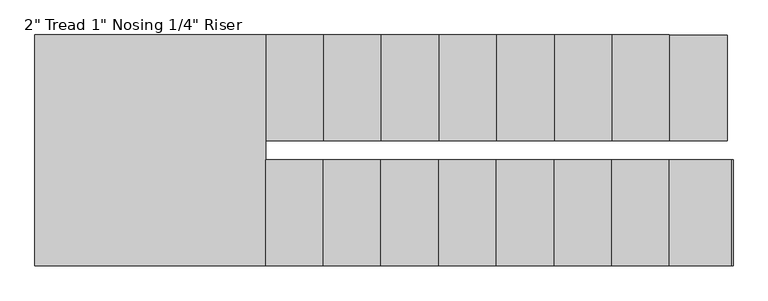
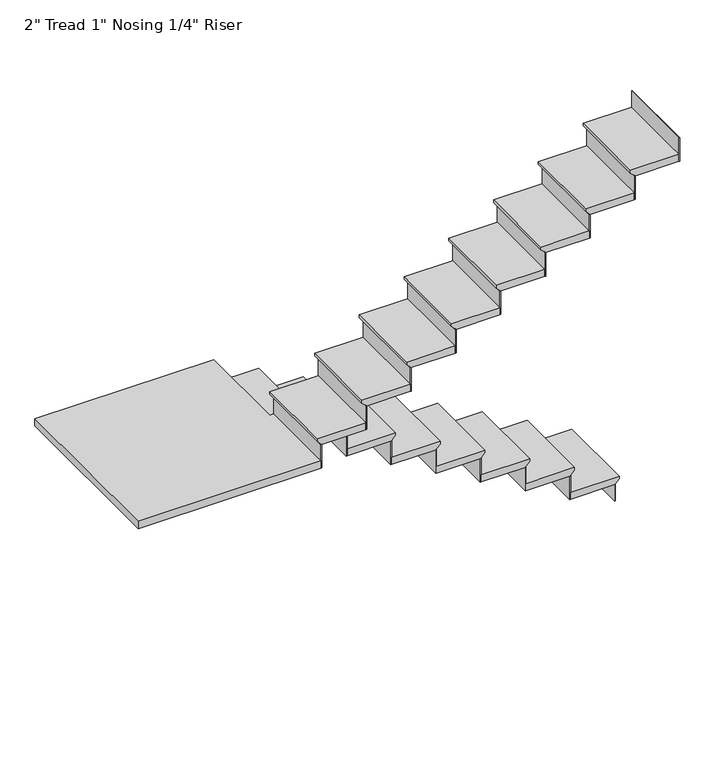
"""IFC4 building model written with IfcOpenShell, lengths in millimetres: stair flight geometry."""

from ifc_helpers import new_model, si_unit, origin, place, context, project, spatial, faceted_brep, source, transform, mapped, element, save


def stair_flight_d84c00c9(model_context):
    return source(origin(), model_context, "Body", "Brep", [
        faceted_brep([(-1805.9198569, -5306.3933037, 9751.4833333), (-1805.9198569, -5306.3933037, 9770.5333333), (-1805.9198569, -5865.1933037, 9770.5333333), (-1805.9198569, -5865.1933037, 9751.4833333), (-1831.3198569, -5306.3933037, 9726.0833333), (-1831.3198569, -5865.1933037, 9726.0833333), (-2136.1198569, -5306.3933037, 9770.5333333), (-2136.1198569, -5865.1933037, 9770.5333333), (-1831.3198569, -5865.1933037, 9719.7333333), (-2136.1198569, -5865.1933037, 9719.7333333), (-2136.1198569, -5306.3933037, 9719.7333333), (-1831.3198569, -5306.3933037, 9719.7333333)], [[[0, 1, 2, 3]], [[4, 0, 3, 5]], [[2, 1, 6, 7]], [[8, 9, 10, 11]], [[2, 7, 9, 8, 5, 3]], [[8, 11, 4, 5]], [[6, 1, 0, 4, 11, 10]], [[7, 6, 10, 9]]]),
        faceted_brep([(-1831.3198569, -5306.3933037, 9719.7333333), (-1831.3198569, -5306.3933037, 9601.2), (-1837.6698569, -5306.3933037, 9601.2), (-1837.6698569, -5306.3933037, 9719.7333333), (-1831.3198569, -5865.1933037, 9719.7333333), (-1837.6698569, -5865.1933037, 9719.7333333), (-1837.6698569, -5865.1933037, 9601.2), (-1831.3198569, -5865.1933037, 9601.2)], [[[0, 1, 2, 3]], [[4, 5, 6, 7]], [[1, 0, 4, 7]], [[2, 1, 7, 6]], [[3, 2, 6, 5]], [[0, 3, 5, 4]]]),
        faceted_brep([(-2136.1198569, -5306.3933037, 9889.0666667), (-2136.1198569, -5306.3933037, 9719.7333333), (-2142.4698569, -5306.3933037, 9719.7333333), (-2142.4698569, -5306.3933037, 9889.0666667), (-2136.1198569, -5865.1933037, 9889.0666667), (-2142.4698569, -5865.1933037, 9889.0666667), (-2142.4698569, -5865.1933037, 9719.7333333), (-2136.1198569, -5865.1933037, 9719.7333333)], [[[0, 1, 2, 3]], [[4, 5, 6, 7]], [[1, 0, 4, 7]], [[2, 1, 7, 6]], [[3, 2, 6, 5]], [[0, 3, 5, 4]]]),
        faceted_brep([(-2110.7198569, -5865.1933037, 9939.8666667), (-2110.7198569, -5306.3933037, 9939.8666667), (-2440.9198569, -5306.3933037, 9939.8666667), (-2440.9198569, -5865.1933037, 9939.8666667), (-2136.1198569, -5865.1933037, 9889.0666667), (-2440.9198569, -5865.1933037, 9889.0666667), (-2440.9198569, -5306.3933037, 9889.0666667), (-2136.1198569, -5306.3933037, 9889.0666667), (-2136.1198569, -5865.1933037, 9895.4166667), (-2110.7198569, -5865.1933037, 9920.8166667), (-2136.1198569, -5306.3933037, 9895.4166667), (-2110.7198569, -5306.3933037, 9920.8166667)], [[[0, 1, 2, 3]], [[4, 5, 6, 7]], [[0, 3, 5, 4, 8, 9]], [[4, 7, 10, 8]], [[2, 1, 11, 10, 7, 6]], [[3, 2, 6, 5]], [[11, 1, 0, 9]], [[10, 11, 9, 8]]]),
        faceted_brep([(-2440.9198569, -5306.3933037, 10058.4), (-2440.9198569, -5306.3933037, 9889.0666667), (-2447.2698569, -5306.3933037, 9889.0666667), (-2447.2698569, -5306.3933037, 10058.4), (-2440.9198569, -5865.1933037, 10058.4), (-2447.2698569, -5865.1933037, 10058.4), (-2447.2698569, -5865.1933037, 9889.0666667), (-2440.9198569, -5865.1933037, 9889.0666667)], [[[0, 1, 2, 3]], [[4, 5, 6, 7]], [[1, 0, 4, 7]], [[2, 1, 7, 6]], [[3, 2, 6, 5]], [[0, 3, 5, 4]]]),
        faceted_brep([(-2415.5198569, -5865.1933037, 10109.2), (-2415.5198569, -5306.3933037, 10109.2), (-2745.7198569, -5306.3933037, 10109.2), (-2745.7198569, -5865.1933037, 10109.2), (-2440.9198569, -5865.1933037, 10058.4), (-2745.7198569, -5865.1933037, 10058.4), (-2745.7198569, -5306.3933037, 10058.4), (-2440.9198569, -5306.3933037, 10058.4), (-2440.9198569, -5865.1933037, 10064.75), (-2415.5198569, -5865.1933037, 10090.15), (-2440.9198569, -5306.3933037, 10064.75), (-2415.5198569, -5306.3933037, 10090.15)], [[[0, 1, 2, 3]], [[4, 5, 6, 7]], [[0, 3, 5, 4, 8, 9]], [[4, 7, 10, 8]], [[2, 1, 11, 10, 7, 6]], [[3, 2, 6, 5]], [[11, 1, 0, 9]], [[10, 11, 9, 8]]]),
        faceted_brep([(-2745.7198569, -5306.3933037, 10227.7333333), (-2745.7198569, -5306.3933037, 10058.4), (-2752.0698569, -5306.3933037, 10058.4), (-2752.0698569, -5306.3933037, 10227.7333333), (-2745.7198569, -5865.1933037, 10227.7333333), (-2752.0698569, -5865.1933037, 10227.7333333), (-2752.0698569, -5865.1933037, 10058.4), (-2745.7198569, -5865.1933037, 10058.4)], [[[0, 1, 2, 3]], [[4, 5, 6, 7]], [[1, 0, 4, 7]], [[2, 1, 7, 6]], [[3, 2, 6, 5]], [[0, 3, 5, 4]]]),
        faceted_brep([(-2720.3198569, -5865.1933037, 10278.5333333), (-2720.3198569, -5306.3933037, 10278.5333333), (-3050.5198569, -5306.3933037, 10278.5333333), (-3050.5198569, -5865.1933037, 10278.5333333), (-2745.7198569, -5865.1933037, 10227.7333333), (-3050.5198569, -5865.1933037, 10227.7333333), (-3050.5198569, -5306.3933037, 10227.7333333), (-2745.7198569, -5306.3933037, 10227.7333333), (-2745.7198569, -5865.1933037, 10234.0833333), (-2720.3198569, -5865.1933037, 10259.4833333), (-2745.7198569, -5306.3933037, 10234.0833333), (-2720.3198569, -5306.3933037, 10259.4833333)], [[[0, 1, 2, 3]], [[4, 5, 6, 7]], [[0, 3, 5, 4, 8, 9]], [[4, 7, 10, 8]], [[2, 1, 11, 10, 7, 6]], [[3, 2, 6, 5]], [[11, 1, 0, 9]], [[10, 11, 9, 8]]]),
        faceted_brep([(-3050.5198569, -5306.3933037, 10397.0666667), (-3050.5198569, -5306.3933037, 10227.7333333), (-3056.8698569, -5306.3933037, 10227.7333333), (-3056.8698569, -5306.3933037, 10397.0666667), (-3050.5198569, -5865.1933037, 10397.0666667), (-3056.8698569, -5865.1933037, 10397.0666667), (-3056.8698569, -5865.1933037, 10227.7333333), (-3050.5198569, -5865.1933037, 10227.7333333)], [[[0, 1, 2, 3]], [[4, 5, 6, 7]], [[1, 0, 4, 7]], [[2, 1, 7, 6]], [[3, 2, 6, 5]], [[0, 3, 5, 4]]]),
        faceted_brep([(-3025.1198569, -5865.1933037, 10447.8666667), (-3025.1198569, -5306.3933037, 10447.8666667), (-3355.3198569, -5306.3933037, 10447.8666667), (-3355.3198569, -5865.1933037, 10447.8666667), (-3050.5198569, -5865.1933037, 10397.0666667), (-3355.3198569, -5865.1933037, 10397.0666667), (-3355.3198569, -5306.3933037, 10397.0666667), (-3050.5198569, -5306.3933037, 10397.0666667), (-3050.5198569, -5865.1933037, 10403.4166667), (-3025.1198569, -5865.1933037, 10428.8166667), (-3050.5198569, -5306.3933037, 10403.4166667), (-3025.1198569, -5306.3933037, 10428.8166667)], [[[0, 1, 2, 3]], [[4, 5, 6, 7]], [[0, 3, 5, 4, 8, 9]], [[4, 7, 10, 8]], [[2, 1, 11, 10, 7, 6]], [[3, 2, 6, 5]], [[11, 1, 0, 9]], [[10, 11, 9, 8]]]),
        faceted_brep([(-3355.3198569, -5306.3933037, 10566.4), (-3355.3198569, -5306.3933037, 10397.0666667), (-3361.6698569, -5306.3933037, 10397.0666667), (-3361.6698569, -5306.3933037, 10566.4), (-3355.3198569, -5865.1933037, 10566.4), (-3361.6698569, -5865.1933037, 10566.4), (-3361.6698569, -5865.1933037, 10397.0666667), (-3355.3198569, -5865.1933037, 10397.0666667)], [[[0, 1, 2, 3]], [[4, 5, 6, 7]], [[1, 0, 4, 7]], [[2, 1, 7, 6]], [[3, 2, 6, 5]], [[0, 3, 5, 4]]]),
        faceted_brep([(-3329.9198569, -5865.1933037, 10617.2), (-3329.9198569, -5306.3933037, 10617.2), (-3660.1198569, -5306.3933037, 10617.2), (-3660.1198569, -5865.1933037, 10617.2), (-3355.3198569, -5865.1933037, 10566.4), (-3660.1198569, -5865.1933037, 10566.4), (-3660.1198569, -5306.3933037, 10566.4), (-3355.3198569, -5306.3933037, 10566.4), (-3355.3198569, -5865.1933037, 10572.75), (-3329.9198569, -5865.1933037, 10598.15), (-3355.3198569, -5306.3933037, 10572.75), (-3329.9198569, -5306.3933037, 10598.15)], [[[0, 1, 2, 3]], [[4, 5, 6, 7]], [[0, 3, 5, 4, 8, 9]], [[4, 7, 10, 8]], [[2, 1, 11, 10, 7, 6]], [[3, 2, 6, 5]], [[11, 1, 0, 9]], [[10, 11, 9, 8]]]),
        faceted_brep([(-3660.1198569, -5306.3933037, 10735.7333333), (-3660.1198569, -5306.3933037, 10566.4), (-3666.4698569, -5306.3933037, 10566.4), (-3666.4698569, -5306.3933037, 10735.7333333), (-3660.1198569, -5865.1933037, 10735.7333333), (-3666.4698569, -5865.1933037, 10735.7333333), (-3666.4698569, -5865.1933037, 10566.4), (-3660.1198569, -5865.1933037, 10566.4)], [[[0, 1, 2, 3]], [[4, 5, 6, 7]], [[1, 0, 4, 7]], [[2, 1, 7, 6]], [[3, 2, 6, 5]], [[0, 3, 5, 4]]]),
        faceted_brep([(-3634.7198569, -5865.1933037, 10786.5333333), (-3634.7198569, -5306.3933037, 10786.5333333), (-3964.9198569, -5306.3933037, 10786.5333333), (-3964.9198569, -5865.1933037, 10786.5333333), (-3660.1198569, -5865.1933037, 10735.7333333), (-3964.9198569, -5865.1933037, 10735.7333333), (-3964.9198569, -5306.3933037, 10735.7333333), (-3660.1198569, -5306.3933037, 10735.7333333), (-3660.1198569, -5865.1933037, 10742.0833333), (-3634.7198569, -5865.1933037, 10767.4833333), (-3660.1198569, -5306.3933037, 10742.0833333), (-3634.7198569, -5306.3933037, 10767.4833333)], [[[0, 1, 2, 3]], [[4, 5, 6, 7]], [[0, 3, 5, 4, 8, 9]], [[4, 7, 10, 8]], [[2, 1, 11, 10, 7, 6]], [[3, 2, 6, 5]], [[11, 1, 0, 9]], [[10, 11, 9, 8]]]),
        faceted_brep([(-3964.9198569, -5306.3933037, 10905.0666667), (-3964.9198569, -5306.3933037, 10735.7333333), (-3971.2698569, -5306.3933037, 10735.7333333), (-3971.2698569, -5306.3933037, 10905.0666667), (-3964.9198569, -5865.1933037, 10905.0666667), (-3971.2698569, -5865.1933037, 10905.0666667), (-3971.2698569, -5865.1933037, 10735.7333333), (-3964.9198569, -5865.1933037, 10735.7333333)], [[[0, 1, 2, 3]], [[4, 5, 6, 7]], [[1, 0, 4, 7]], [[2, 1, 7, 6]], [[3, 2, 6, 5]], [[0, 3, 5, 4]]]),
        faceted_brep([(-3939.5198569, -5865.1933037, 10955.8666667), (-3939.5198569, -5306.3933037, 10955.8666667), (-4269.7198569, -5306.3933037, 10955.8666667), (-4269.7198569, -5865.1933037, 10955.8666667), (-3964.9198569, -5865.1933037, 10905.0666667), (-4269.7198569, -5865.1933037, 10905.0666667), (-4269.7198569, -5306.3933037, 10905.0666667), (-3964.9198569, -5306.3933037, 10905.0666667), (-3964.9198569, -5865.1933037, 10911.4166667), (-3939.5198569, -5865.1933037, 10936.8166667), (-3964.9198569, -5306.3933037, 10911.4166667), (-3939.5198569, -5306.3933037, 10936.8166667)], [[[0, 1, 2, 3]], [[4, 5, 6, 7]], [[0, 3, 5, 4, 8, 9]], [[4, 7, 10, 8]], [[2, 1, 11, 10, 7, 6]], [[3, 2, 6, 5]], [[11, 1, 0, 9]], [[10, 11, 9, 8]]]),
        faceted_brep([(-4269.7198569, -5306.3933037, 11074.4), (-4269.7198569, -5306.3933037, 10905.0666667), (-4276.0698569, -5306.3933037, 10905.0666667), (-4276.0698569, -5306.3933037, 11074.4), (-4269.7198569, -5865.1933037, 11074.4), (-4276.0698569, -5865.1933037, 11074.4), (-4276.0698569, -5865.1933037, 10905.0666667), (-4269.7198569, -5865.1933037, 10905.0666667)], [[[0, 1, 2, 3]], [[4, 5, 6, 7]], [[1, 0, 4, 7]], [[2, 1, 7, 6]], [[3, 2, 6, 5]], [[0, 3, 5, 4]]]),
        faceted_brep([(-4218.9198569, -5966.7933037, 11125.2), (-4244.3198569, -5966.7933037, 11125.2), (-4244.3198569, -5306.3933037, 11125.2), (-5463.5198569, -5306.3933037, 11125.2), (-5463.5198569, -6525.5933037, 11125.2), (-4218.9198569, -6525.5933037, 11125.2), (-4244.3198569, -5966.7933037, 11074.4), (-4218.9198569, -5966.7933037, 11074.4), (-4218.9198569, -6525.5933037, 11074.4), (-5463.5198569, -6525.5933037, 11074.4), (-5463.5198569, -5306.3933037, 11074.4), (-4269.7198569, -5306.3933037, 11074.4), (-4269.7198569, -5865.1933037, 11074.4), (-4244.3198569, -5865.1933037, 11074.4), (-4244.3198569, -5865.1933037, 11106.15), (-4244.3198569, -5306.3933037, 11106.15), (-4269.7198569, -5865.1933037, 11080.75), (-4269.7198569, -5306.3933037, 11080.75)], [[[0, 1, 2, 3, 4, 5]], [[6, 7, 8, 9, 10, 11, 12, 13]], [[1, 0, 7, 6]], [[2, 1, 6, 13, 14, 15]], [[13, 12, 16, 14]], [[12, 11, 17, 16]], [[3, 2, 15, 17, 11, 10]], [[4, 3, 10, 9]], [[5, 4, 9, 8]], [[0, 5, 8, 7]], [[17, 15, 14, 16]]]),
        faceted_brep([(-4218.9198569, -6525.5933037, 11243.7333333), (-4218.9198569, -6525.5933037, 11074.4), (-4212.5698569, -6525.5933037, 11074.4), (-4212.5698569, -6525.5933037, 11243.7333333), (-4218.9198569, -5966.7933037, 11243.7333333), (-4212.5698569, -5966.7933037, 11243.7333333), (-4212.5698569, -5966.7933037, 11074.4), (-4218.9198569, -5966.7933037, 11074.4)], [[[0, 1, 2, 3]], [[4, 5, 6, 7]], [[1, 0, 4, 7]], [[2, 1, 7, 6]], [[3, 2, 6, 5]], [[0, 3, 5, 4]]]),
        faceted_brep([(-4244.3198569, -5966.7933037, 11294.5333333), (-4244.3198569, -6525.5933037, 11294.5333333), (-3914.1198569, -6525.5933037, 11294.5333333), (-3914.1198569, -5966.7933037, 11294.5333333), (-4218.9198569, -5966.7933037, 11243.7333333), (-3914.1198569, -5966.7933037, 11243.7333333), (-3914.1198569, -6525.5933037, 11243.7333333), (-4218.9198569, -6525.5933037, 11243.7333333), (-4218.9198569, -5966.7933037, 11250.0833333), (-4244.3198569, -5966.7933037, 11275.4833333), (-4218.9198569, -6525.5933037, 11250.0833333), (-4244.3198569, -6525.5933037, 11275.4833333)], [[[0, 1, 2, 3]], [[4, 5, 6, 7]], [[0, 3, 5, 4, 8, 9]], [[4, 7, 10, 8]], [[2, 1, 11, 10, 7, 6]], [[3, 2, 6, 5]], [[11, 1, 0, 9]], [[10, 11, 9, 8]]]),
        faceted_brep([(-3914.1198569, -6525.5933037, 11413.0666667), (-3914.1198569, -6525.5933037, 11243.7333333), (-3907.7698569, -6525.5933037, 11243.7333333), (-3907.7698569, -6525.5933037, 11413.0666667), (-3914.1198569, -5966.7933037, 11413.0666667), (-3907.7698569, -5966.7933037, 11413.0666667), (-3907.7698569, -5966.7933037, 11243.7333333), (-3914.1198569, -5966.7933037, 11243.7333333)], [[[0, 1, 2, 3]], [[4, 5, 6, 7]], [[1, 0, 4, 7]], [[2, 1, 7, 6]], [[3, 2, 6, 5]], [[0, 3, 5, 4]]]),
        faceted_brep([(-3939.5198569, -5966.7933037, 11463.8666667), (-3939.5198569, -6525.5933037, 11463.8666667), (-3609.3198569, -6525.5933037, 11463.8666667), (-3609.3198569, -5966.7933037, 11463.8666667), (-3914.1198569, -5966.7933037, 11413.0666667), (-3609.3198569, -5966.7933037, 11413.0666667), (-3609.3198569, -6525.5933037, 11413.0666667), (-3914.1198569, -6525.5933037, 11413.0666667), (-3914.1198569, -5966.7933037, 11419.4166667), (-3939.5198569, -5966.7933037, 11444.8166667), (-3914.1198569, -6525.5933037, 11419.4166667), (-3939.5198569, -6525.5933037, 11444.8166667)], [[[0, 1, 2, 3]], [[4, 5, 6, 7]], [[0, 3, 5, 4, 8, 9]], [[4, 7, 10, 8]], [[2, 1, 11, 10, 7, 6]], [[3, 2, 6, 5]], [[11, 1, 0, 9]], [[10, 11, 9, 8]]]),
        faceted_brep([(-3609.3198569, -6525.5933037, 11582.4), (-3609.3198569, -6525.5933037, 11413.0666667), (-3602.9698569, -6525.5933037, 11413.0666667), (-3602.9698569, -6525.5933037, 11582.4), (-3609.3198569, -5966.7933037, 11582.4), (-3602.9698569, -5966.7933037, 11582.4), (-3602.9698569, -5966.7933037, 11413.0666667), (-3609.3198569, -5966.7933037, 11413.0666667)], [[[0, 1, 2, 3]], [[4, 5, 6, 7]], [[1, 0, 4, 7]], [[2, 1, 7, 6]], [[3, 2, 6, 5]], [[0, 3, 5, 4]]]),
        faceted_brep([(-3634.7198569, -5966.7933037, 11633.2), (-3634.7198569, -6525.5933037, 11633.2), (-3304.5198569, -6525.5933037, 11633.2), (-3304.5198569, -5966.7933037, 11633.2), (-3609.3198569, -5966.7933037, 11582.4), (-3304.5198569, -5966.7933037, 11582.4), (-3304.5198569, -6525.5933037, 11582.4), (-3609.3198569, -6525.5933037, 11582.4), (-3609.3198569, -5966.7933037, 11588.75), (-3634.7198569, -5966.7933037, 11614.15), (-3609.3198569, -6525.5933037, 11588.75), (-3634.7198569, -6525.5933037, 11614.15)], [[[0, 1, 2, 3]], [[4, 5, 6, 7]], [[0, 3, 5, 4, 8, 9]], [[4, 7, 10, 8]], [[2, 1, 11, 10, 7, 6]], [[3, 2, 6, 5]], [[11, 1, 0, 9]], [[10, 11, 9, 8]]]),
        faceted_brep([(-3304.5198569, -6525.5933037, 11751.7333333), (-3304.5198569, -6525.5933037, 11582.4), (-3298.1698569, -6525.5933037, 11582.4), (-3298.1698569, -6525.5933037, 11751.7333333), (-3304.5198569, -5966.7933037, 11751.7333333), (-3298.1698569, -5966.7933037, 11751.7333333), (-3298.1698569, -5966.7933037, 11582.4), (-3304.5198569, -5966.7933037, 11582.4)], [[[0, 1, 2, 3]], [[4, 5, 6, 7]], [[1, 0, 4, 7]], [[2, 1, 7, 6]], [[3, 2, 6, 5]], [[0, 3, 5, 4]]]),
        faceted_brep([(-3329.9198569, -5966.7933037, 11802.5333333), (-3329.9198569, -6525.5933037, 11802.5333333), (-2999.7198569, -6525.5933037, 11802.5333333), (-2999.7198569, -5966.7933037, 11802.5333333), (-3304.5198569, -5966.7933037, 11751.7333333), (-2999.7198569, -5966.7933037, 11751.7333333), (-2999.7198569, -6525.5933037, 11751.7333333), (-3304.5198569, -6525.5933037, 11751.7333333), (-3304.5198569, -5966.7933037, 11758.0833333), (-3329.9198569, -5966.7933037, 11783.4833333), (-3304.5198569, -6525.5933037, 11758.0833333), (-3329.9198569, -6525.5933037, 11783.4833333)], [[[0, 1, 2, 3]], [[4, 5, 6, 7]], [[0, 3, 5, 4, 8, 9]], [[4, 7, 10, 8]], [[2, 1, 11, 10, 7, 6]], [[3, 2, 6, 5]], [[11, 1, 0, 9]], [[10, 11, 9, 8]]]),
        faceted_brep([(-2999.7198569, -6525.5933037, 11921.0666667), (-2999.7198569, -6525.5933037, 11751.7333333), (-2993.3698569, -6525.5933037, 11751.7333333), (-2993.3698569, -6525.5933037, 11921.0666667), (-2999.7198569, -5966.7933037, 11921.0666667), (-2993.3698569, -5966.7933037, 11921.0666667), (-2993.3698569, -5966.7933037, 11751.7333333), (-2999.7198569, -5966.7933037, 11751.7333333)], [[[0, 1, 2, 3]], [[4, 5, 6, 7]], [[1, 0, 4, 7]], [[2, 1, 7, 6]], [[3, 2, 6, 5]], [[0, 3, 5, 4]]]),
        faceted_brep([(-3025.1198569, -5966.7933037, 11971.8666667), (-3025.1198569, -6525.5933037, 11971.8666667), (-2694.9198569, -6525.5933037, 11971.8666667), (-2694.9198569, -5966.7933037, 11971.8666667), (-2999.7198569, -5966.7933037, 11921.0666667), (-2694.9198569, -5966.7933037, 11921.0666667), (-2694.9198569, -6525.5933037, 11921.0666667), (-2999.7198569, -6525.5933037, 11921.0666667), (-2999.7198569, -5966.7933037, 11927.4166667), (-3025.1198569, -5966.7933037, 11952.8166667), (-2999.7198569, -6525.5933037, 11927.4166667), (-3025.1198569, -6525.5933037, 11952.8166667)], [[[0, 1, 2, 3]], [[4, 5, 6, 7]], [[0, 3, 5, 4, 8, 9]], [[4, 7, 10, 8]], [[2, 1, 11, 10, 7, 6]], [[3, 2, 6, 5]], [[11, 1, 0, 9]], [[10, 11, 9, 8]]]),
        faceted_brep([(-2694.9198569, -6525.5933037, 12090.4), (-2694.9198569, -6525.5933037, 11921.0666667), (-2688.5698569, -6525.5933037, 11921.0666667), (-2688.5698569, -6525.5933037, 12090.4), (-2694.9198569, -5966.7933037, 12090.4), (-2688.5698569, -5966.7933037, 12090.4), (-2688.5698569, -5966.7933037, 11921.0666667), (-2694.9198569, -5966.7933037, 11921.0666667)], [[[0, 1, 2, 3]], [[4, 5, 6, 7]], [[1, 0, 4, 7]], [[2, 1, 7, 6]], [[3, 2, 6, 5]], [[0, 3, 5, 4]]]),
        faceted_brep([(-2720.3198569, -5966.7933037, 12141.2), (-2720.3198569, -6525.5933037, 12141.2), (-2390.1198569, -6525.5933037, 12141.2), (-2390.1198569, -5966.7933037, 12141.2), (-2694.9198569, -5966.7933037, 12090.4), (-2390.1198569, -5966.7933037, 12090.4), (-2390.1198569, -6525.5933037, 12090.4), (-2694.9198569, -6525.5933037, 12090.4), (-2694.9198569, -5966.7933037, 12096.75), (-2720.3198569, -5966.7933037, 12122.15), (-2694.9198569, -6525.5933037, 12096.75), (-2720.3198569, -6525.5933037, 12122.15)], [[[0, 1, 2, 3]], [[4, 5, 6, 7]], [[0, 3, 5, 4, 8, 9]], [[4, 7, 10, 8]], [[2, 1, 11, 10, 7, 6]], [[3, 2, 6, 5]], [[11, 1, 0, 9]], [[10, 11, 9, 8]]]),
        faceted_brep([(-2390.1198569, -6525.5933037, 12259.7333333), (-2390.1198569, -6525.5933037, 12090.4), (-2383.7698569, -6525.5933037, 12090.4), (-2383.7698569, -6525.5933037, 12259.7333333), (-2390.1198569, -5966.7933037, 12259.7333333), (-2383.7698569, -5966.7933037, 12259.7333333), (-2383.7698569, -5966.7933037, 12090.4), (-2390.1198569, -5966.7933037, 12090.4)], [[[0, 1, 2, 3]], [[4, 5, 6, 7]], [[1, 0, 4, 7]], [[2, 1, 7, 6]], [[3, 2, 6, 5]], [[0, 3, 5, 4]]]),
        faceted_brep([(-2415.5198569, -5966.7933037, 12310.5333333), (-2415.5198569, -6525.5933037, 12310.5333333), (-2085.3198569, -6525.5933037, 12310.5333333), (-2085.3198569, -5966.7933037, 12310.5333333), (-2390.1198569, -5966.7933037, 12259.7333333), (-2085.3198569, -5966.7933037, 12259.7333333), (-2085.3198569, -6525.5933037, 12259.7333333), (-2390.1198569, -6525.5933037, 12259.7333333), (-2390.1198569, -5966.7933037, 12266.0833333), (-2415.5198569, -5966.7933037, 12291.4833333), (-2390.1198569, -6525.5933037, 12266.0833333), (-2415.5198569, -6525.5933037, 12291.4833333)], [[[0, 1, 2, 3]], [[4, 5, 6, 7]], [[0, 3, 5, 4, 8, 9]], [[4, 7, 10, 8]], [[2, 1, 11, 10, 7, 6]], [[3, 2, 6, 5]], [[11, 1, 0, 9]], [[10, 11, 9, 8]]]),
        faceted_brep([(-2085.3198569, -6525.5933037, 12429.0666667), (-2085.3198569, -6525.5933037, 12259.7333333), (-2078.9698569, -6525.5933037, 12259.7333333), (-2078.9698569, -6525.5933037, 12429.0666667), (-2085.3198569, -5966.7933037, 12429.0666667), (-2078.9698569, -5966.7933037, 12429.0666667), (-2078.9698569, -5966.7933037, 12259.7333333), (-2085.3198569, -5966.7933037, 12259.7333333)], [[[0, 1, 2, 3]], [[4, 5, 6, 7]], [[1, 0, 4, 7]], [[2, 1, 7, 6]], [[3, 2, 6, 5]], [[0, 3, 5, 4]]]),
        faceted_brep([(-1780.5198569, -6525.5933037, 12598.4), (-1780.5198569, -6525.5933037, 12429.0666667), (-1774.1698569, -6525.5933037, 12429.0666667), (-1774.1698569, -6525.5933037, 12598.4), (-1780.5198569, -5966.7933037, 12598.4), (-1774.1698569, -5966.7933037, 12598.4), (-1774.1698569, -5966.7933037, 12429.0666667), (-1780.5198569, -5966.7933037, 12429.0666667)], [[[0, 1, 2, 3]], [[4, 5, 6, 7]], [[1, 0, 4, 7]], [[2, 1, 7, 6]], [[3, 2, 6, 5]], [[0, 3, 5, 4]]]),
        faceted_brep([(-2110.7198569, -5966.7933037, 12479.8666667), (-2110.7198569, -6525.5933037, 12479.8666667), (-1780.5198569, -6525.5933037, 12479.8666667), (-1780.5198569, -5966.7933037, 12479.8666667), (-2085.3198569, -5966.7933037, 12429.0666667), (-1780.5198569, -5966.7933037, 12429.0666667), (-1780.5198569, -6525.5933037, 12429.0666667), (-2085.3198569, -6525.5933037, 12429.0666667), (-2085.3198569, -5966.7933037, 12435.4166667), (-2110.7198569, -5966.7933037, 12460.8166667), (-2085.3198569, -6525.5933037, 12435.4166667), (-2110.7198569, -6525.5933037, 12460.8166667)], [[[0, 1, 2, 3]], [[4, 5, 6, 7]], [[0, 3, 5, 4, 8, 9]], [[4, 7, 10, 8]], [[2, 1, 11, 10, 7, 6]], [[3, 2, 6, 5]], [[11, 1, 0, 9]], [[10, 11, 9, 8]]]),
    ])


if __name__ == "__main__":
    model = new_model("IFC4")
    model_context = context("Model", 3, world=origin())
    ifc_project = project(units=[si_unit("LENGTHUNIT", "METRE", prefix="MILLI")], contexts=[model_context])
    site = spatial("IfcSite", under=ifc_project)
    building = spatial("IfcBuilding", under=site)
    placement = place(None, origin())
    stair_flight_shape = stair_flight_d84c00c9(model_context)
    element("IfcStairFlight", 1, ObjectType="2\" Tread 1\" Nosing 1/4\" Riser", at=placement, inside=building, context=model_context, shape_type="MappedRepresentation", body=[
        mapped(stair_flight_shape, transform((0.0, 0.0, 0.0), x_axis=(1.0, 0.0, 0.0), y_axis=(0.0, 1.0, 0.0), z_axis=(0.0, 0.0, 1.0))),
    ])
    save(model, "model.ifc")
